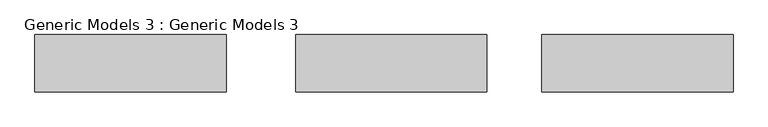
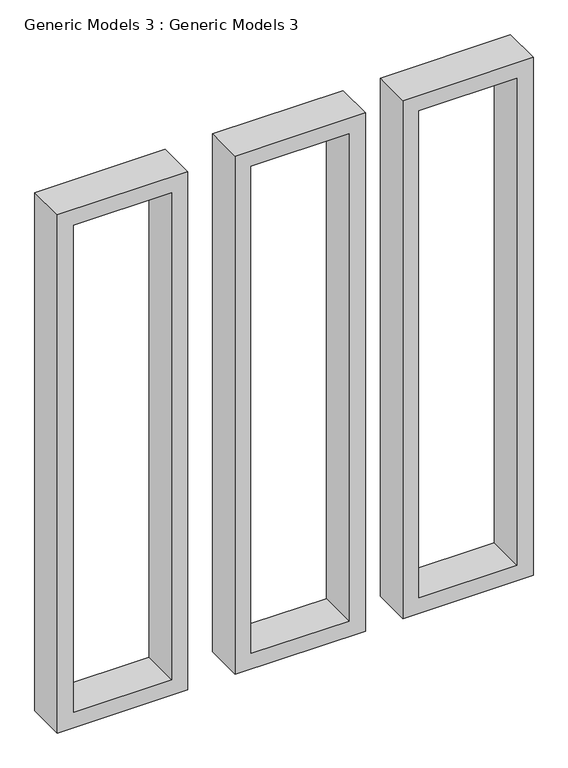
"""IFC4 building model written with IfcOpenShell, lengths in millimetres: proxy geometry, Generic Models 3 : Generic Models 3."""

from ifc_helpers import new_model, si_unit, frame, origin, place, context, project, spatial, polyline, outline, extrude, source, transform, mapped, element, save


def generic_models_3_generic_models_3_7aa97fcf(model_context):
    return source(origin(), model_context, "Body", "SweptSolid", [
        extrude(outline(polyline([(3657.6, -7968.2171142), (3657.6, -7460.2171142), (5791.2, -7460.2171142), (5791.2, -7968.2171142), (3657.6, -7968.2171142)]), holes=[polyline([(3721.1, -7904.7171142), (5727.7, -7904.7171142), (5727.7, -7523.7171142), (3721.1, -7523.7171142), (3721.1, -7904.7171142)])]), frame((0.0, -12161.7509606, 0.0), z_axis=(0.0, 1.0, 0.0), x_axis=(0.0, 0.0, 1.0)), (0.0, 0.0, 1.0), 152.4),
        extrude(outline(polyline([(3657.6, -7276.0671142), (3657.6, -6768.0671142), (5791.2, -6768.0671142), (5791.2, -7276.0671142), (3657.6, -7276.0671142)]), holes=[polyline([(3721.1, -7212.5671142), (5727.7, -7212.5671142), (5727.7, -6831.5671142), (3721.1, -6831.5671142), (3721.1, -7212.5671142)])]), frame((0.0, -12161.7509606, 0.0), z_axis=(0.0, 1.0, 0.0), x_axis=(0.0, 0.0, 1.0)), (0.0, 0.0, 1.0), 152.4),
        extrude(outline(polyline([(3657.6, -6622.0171142), (3657.6, -6114.0171142), (5791.2, -6114.0171142), (5791.2, -6622.0171142), (3657.6, -6622.0171142)]), holes=[polyline([(3721.1, -6558.5171142), (5727.7, -6558.5171142), (5727.7, -6177.5171142), (3721.1, -6177.5171142), (3721.1, -6558.5171142)])]), frame((0.0, -12161.7509606, 0.0), z_axis=(0.0, 1.0, 0.0), x_axis=(0.0, 0.0, 1.0)), (0.0, 0.0, 1.0), 152.4),
    ])


if __name__ == "__main__":
    model = new_model("IFC4")
    model_context = context("Model", 3, world=origin())
    ifc_project = project(units=[si_unit("LENGTHUNIT", "METRE", prefix="MILLI")], contexts=[model_context])
    site = spatial("IfcSite", under=ifc_project)
    building = spatial("IfcBuilding", under=site)
    placement = place(None, origin())
    generic_models_3_generic_models_3_shape = generic_models_3_generic_models_3_7aa97fcf(model_context)
    element("IfcBuildingElementProxy", 1, Name="Generic Models 3 : Generic Models 3", ObjectType="Generic Models 3 : Generic Models 3", at=placement, inside=building, context=model_context, shape_type="MappedRepresentation", body=[
        mapped(generic_models_3_generic_models_3_shape, transform((0.0, 0.0, 0.0), x_axis=(1.0, 0.0, 0.0), y_axis=(0.0, 1.0, 0.0), z_axis=(0.0, 0.0, 1.0))),
    ])
    save(model, "model.ifc")

# Revit data of these elements
# Element 1 (IfcBuildingElementProxy, "Generic Models 3 : Generic Models 3")
#   Materials on its faces: "GREY COLOUR FRAME(1)"
# Materials
#   "GREY COLOUR FRAME(1)": class "Generic", colour RGB 120 120 120, transparency 0, Cost = 0
